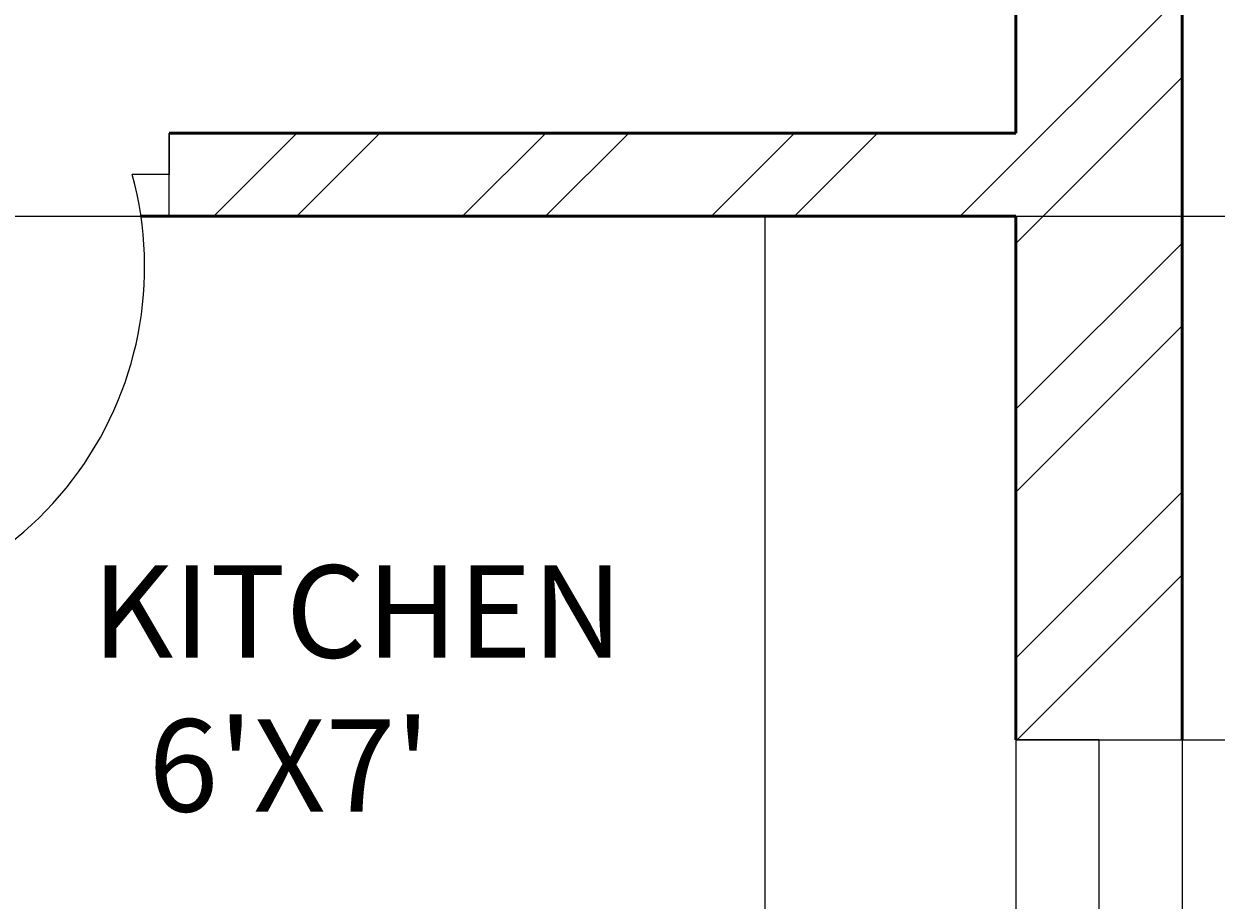
# Model space of a CAD drawing. Units: inches. Extents: x 2310 to 2937, y 1113 to 2410.
# Tile 13 of 23: x 2761 to 2826, y 1845 to 1893. Entities that reach past the tile are written whole.
import ezdxf

# ---------------------------------------------------------------- set-up
doc = ezdxf.new("R2010")
doc.units = ezdxf.units.IN
for name, color, linetype, lineweight in [('A-ANNO-DIMS', 2, 'Continuous', 18), ('A-AREA-IDEN', 7, 'Continuous', 18), ('A-DOOR', 31, 'Continuous', 25), ('A-FLOR-CASE', 7, 'Continuous', 25), ('A-GLAZ', 191, 'Continuous', 20), ('A-WALL', 7, 'Continuous', 50), ('A-WALL-PATT', 85, 'Continuous', 13)]:
    doc.layers.add(name, color=color, linetype=linetype, lineweight=lineweight)
doc.styles.get("Standard").update_dxf_attribs({"font": 'arial.ttf'})
doc.dimstyles.get("Standard").update_dxf_attribs({"dimtxt": 0.18, "dimasz": 0.18, "dimexe": 0.18, "dimexo": 0.0625, "dimgap": 0.09, "dimtad": 0, "dimtih": 1, "dimtoh": 1, "dimdec": 4, "dimzin": 0, "dimdsep": 46, "dimtxsty": 'Standard', "dimcen": 0.09, "dimadec": 0, "dimazin": 0, "dimtfac": 1, "dimtdec": 4, "dimtofl": 0, "dimtmove": 0, "dimatfit": 3, "dimfxl": 1, "dimtolj": 1, "dimtzin": 0, "dimarcsym": 0})

# ---------------------------------------------------------------- blocks, each defined once
blk = doc.blocks.new('WIN-36IN')
for p, q in [((4.5, 36), (0, 36)), ((0, 36), (9, 36)), ((0, 36), (0, 0)), ((4.5, 0), (4.5, 36)), ((9, 36), (9, 0)), ((0, 0), (9, 0)), ((9, 0), (4.5, 0))]:
    blk.add_line(p, q)
blk = doc.blocks.new('*D47')
at = {"layer": 'A-ANNO-DIMS', "color": 0, "lineweight": -2, "transparency": 16777216}
for p, q in [((2824.048, 1909.978), (2858.016, 1909.978)), ((2857.836, 1909.798), (2857.836, 1882.256)), ((2857.836, 1854.35), (2857.836, 1881.893)), ((2824.048, 1854.17), (2858.016, 1854.17))]:
    blk.add_line(p, q, dxfattribs=at)
at = {"layer": 'A-ANNO-DIMS', "color": 0, "transparency": 16777216}
for points in [[(2857.806, 1909.798), (2857.866, 1909.798), (2857.836, 1909.978)], [(2857.806, 1854.35), (2857.866, 1854.35), (2857.836, 1854.17)]]:
    blk.add_solid(points, dxfattribs=at)
at = {"layer": 'Defpoints', "color": 0, "transparency": 16777216}
for p in [(2823.986, 1909.978), (2857.836, 1909.978), (2823.986, 1854.17)]:
    blk.add_point(p, dxfattribs=at)
at = {"layer": 'A-ANNO-DIMS', "color": 0, "transparency": 16777216, "insert": (2857.836, 1882.074), "char_height": 0.18, "attachment_point": 5}
blk.add_mtext('\\A1;55.81', dxfattribs=at)
blk = doc.blocks.new('*D58')
at = {"layer": 'A-ANNO-DIMS', "color": 0, "lineweight": -2, "transparency": 16777216}
for p, q in [((2475.548, 1882.514), (2858.016, 1882.514)), ((2857.836, 1882.334), (2857.836, 1840.446)), ((2857.836, 1798.194), (2857.836, 1840.082)), ((2475.548, 1798.014), (2858.016, 1798.014))]:
    blk.add_line(p, q, dxfattribs=at)
at = {"layer": 'A-ANNO-DIMS', "color": 0, "transparency": 16777216}
for points in [[(2857.806, 1882.334), (2857.866, 1882.334), (2857.836, 1882.514)], [(2857.806, 1798.194), (2857.866, 1798.194), (2857.836, 1798.014)]]:
    blk.add_solid(points, dxfattribs=at)
at = {"layer": 'Defpoints', "color": 0, "transparency": 16777216}
for p in [(2475.486, 1882.514), (2857.836, 1882.514), (2475.486, 1798.014)]:
    blk.add_point(p, dxfattribs=at)
at = {"layer": 'A-ANNO-DIMS', "color": 0, "transparency": 16777216, "insert": (2857.836, 1840.264), "char_height": 0.18, "attachment_point": 5}
blk.add_mtext('\\A1;84.5', dxfattribs=at)

msp = doc.modelspace()

# ---------------------------------------------------------------- hatches: boundary and pattern name
at = {"layer": 'A-WALL-PATT'}
h = msp.add_hatch(dxfattribs=at)
h.set_pattern_fill('ANSI32', color=256)
h.paths.add_polyline_path([(2639.1394, 2356.5139), (2563.662, 2356.5139), (2563.662, 2347.5139), (2606.9859, 2347.5139), (2606.9859, 2210.5139), (2514.2692, 2210.5139), (2514.2692, 2206.0139), (2606.9859, 2206.0139), (2606.9859, 2098.0139), (2602.689, 2098.0139), (2602.689, 2093.5139), (2615.5262, 2093.5139), (2615.5262, 2095.7639), (2615.5262, 2098.0139), (2611.4859, 2098.0139), (2611.4859, 2206.0139), (2703.9391, 2206.0139), (2703.9391, 2208.2639), (2703.9391, 2210.5139), (2611.4859, 2210.5139), (2611.4859, 2347.5139), (2639.1394, 2347.5139)])
h.paths.add_polyline_path([(2823.9859, 2356.5139), (2699.1394, 2356.5139), (2699.1394, 2347.5139), (2738.4859, 2347.5139), (2738.4859, 2343.9266), (2742.9859, 2343.9266), (2742.9859, 2347.5139), (2814.9859, 2347.5139), (2814.9859, 2336.76), (2823.9859, 2336.76)])
h.paths.add_polyline_path([(2823.9859, 2312.76), (2814.9859, 2312.76), (2814.9859, 2299.5139), (2742.9859, 2299.5139), (2742.9859, 2323.0159), (2740.7359, 2323.0159), (2738.4859, 2323.0159), (2738.4859, 2210.5139), (2734.5483, 2210.5139), (2734.5483, 2206.0139), (2746.8769, 2206.0139), (2746.8769, 2208.2639), (2746.8769, 2210.5139), (2742.9859, 2210.5139), (2742.9859, 2295.0139), (2814.9859, 2295.0139), (2814.9859, 2269.8977), (2823.9859, 2269.8977)])
h.paths.add_polyline_path([(2823.9859, 2210.5139), (2823.9859, 2233.8977), (2819.4859, 2233.8977), (2814.9859, 2233.8977), (2814.9859, 2210.5139), (2769.9745, 2210.5139), (2769.9745, 2206.0139), (2814.9859, 2206.0139), (2814.9859, 2178.3027), (2823.9859, 2178.3027)])
h.paths.add_polyline_path([(2823.9859, 2118.3027), (2819.4859, 2118.3027), (2814.9859, 2118.3027), (2814.9859, 2098.0139), (2647.0333, 2098.0139), (2647.0333, 2093.5139), (2814.9859, 2093.5139), (2814.9859, 1999.5139), (2650.6052, 1999.5139), (2650.6052, 1995.0139), (2814.9859, 1995.0139), (2814.9859, 1969.9784), (2823.9859, 1969.9784)])
h.paths.add_polyline_path([(2403.4859, 2093.5139), (2569.9888, 2093.5139), (2569.9888, 2095.7639), (2569.9888, 2098.0139), (2403.4859, 2098.0139), (2403.4859, 2131.7587), (2394.4859, 2131.7587), (2394.4859, 1967.522), (2403.4859, 1967.522), (2403.4859, 1995.0139), (2569.8903, 1995.0139), (2569.8903, 1997.2639), (2569.8903, 1999.5139), (2403.4859, 1999.5139)])
h.paths.add_polyline_path([(2503.662, 2356.5139), (2394.4859, 2356.5139), (2394.4859, 2337.9231), (2398.9859, 2337.9231), (2403.4859, 2337.9231), (2403.4859, 2347.5139), (2475.4859, 2347.5139), (2475.4859, 2343.0384), (2479.9859, 2343.0384), (2479.9859, 2347.5139), (2503.662, 2347.5139)])
h.paths.add_polyline_path([(2498.3065, 1745.5139), (2479.9859, 1745.5139), (2479.9859, 1749.1663), (2477.7359, 1749.1663), (2475.4859, 1749.1663), (2475.4859, 1745.5139), (2403.4859, 1745.5139), (2403.4859, 1753.6409), (2398.9859, 1753.6409), (2394.4859, 1753.6409), (2394.4859, 1736.5139), (2498.3065, 1736.5139), (2498.3065, 1741.0139)])
h.paths.add_polyline_path([(2479.9859, 1882.5139), (2483.9367, 1882.5139), (2483.9367, 1887.0139), (2471.5501, 1887.0139), (2471.5501, 1885.1969), (2471.5501, 1882.5139), (2475.4859, 1882.5139), (2475.4859, 1798.0139), (2403.4859, 1798.0139), (2403.4859, 1828.0433), (2402.2852, 1828.0433), (2394.4859, 1828.0433), (2394.4859, 1777.6409), (2403.4859, 1777.6409), (2403.4859, 1793.5139), (2475.4859, 1793.5139), (2475.4859, 1769.1696), (2479.9859, 1769.1696)])
h.paths.add_polyline_path([(2403.4859, 1907.522), (2398.9859, 1907.522), (2394.4859, 1907.522), (2394.4859, 1864.0433), (2403.4859, 1864.0433), (2403.4859, 1882.5139), (2448.9325, 1882.5139), (2448.9325, 1884.7639), (2448.9325, 1887.0139), (2403.4859, 1887.0139)])
h.paths.add_polyline_path([(2702.2061, 1887.0139), (2611.4859, 1887.0139), (2611.4859, 1995.0139), (2615.6132, 1995.0139), (2615.6132, 1999.5139), (2602.4798, 1999.5139), (2602.4798, 1997.2639), (2602.4798, 1995.0139), (2606.9859, 1995.0139), (2606.9859, 1887.0139), (2516.2443, 1887.0139), (2516.2443, 1884.7639), (2516.2443, 1882.5139), (2606.9859, 1882.5139), (2606.9859, 1745.5139), (2558.3065, 1745.5139), (2558.3065, 1736.5139), (2638.8921, 1736.5139), (2638.8921, 1741.0139), (2638.8921, 1745.5139), (2611.4859, 1745.5139), (2611.4859, 1882.5139), (2702.2061, 1882.5139)])
h.paths.add_polyline_path([(2823.9859, 1909.9784), (2819.4859, 1909.9784), (2814.9859, 1909.9784), (2814.9859, 1887.0139), (2769.144, 1887.0139), (2769.144, 1884.7639), (2769.144, 1882.5139), (2814.9859, 1882.5139), (2814.9859, 1854.1704), (2823.9859, 1854.1704)])
h.paths.add_polyline_path([(2823.9859, 1818.1704), (2819.4859, 1818.1704), (2814.9859, 1818.1704), (2814.9859, 1798.0139), (2742.9859, 1798.0139), (2742.9859, 1882.5139), (2746.805, 1882.5139), (2746.805, 1887.0139), (2733.7334, 1887.0139), (2733.7334, 1884.7639), (2733.7334, 1882.5139), (2738.4859, 1882.5139), (2738.4859, 1771.1728), (2740.7359, 1771.1728), (2742.9859, 1771.1728), (2742.9859, 1793.5139), (2814.9859, 1793.5139), (2814.9859, 1783.6684), (2823.9859, 1783.6684)])
h.paths.add_polyline_path([(2823.9859, 1759.6684), (2814.9859, 1759.6684), (2814.9859, 1745.5139), (2742.9859, 1745.5139), (2742.9859, 1748.9831), (2740.7359, 1748.9831), (2738.4859, 1748.9831), (2738.4859, 1745.5139), (2698.8921, 1745.5139), (2698.8921, 1736.5139), (2823.9859, 1736.5139)])

# ---------------------------------------------------------------- linework, layer by layer
at = {"layer": 'A-DOOR'}
for p, q in [((2769.144, 1882.5139), (2769.144, 1887.0139)), ((2769.144, 1887.0139), (2769.144, 1884.7639)), ((2769.144, 1884.7639), (2767.144, 1884.7639))]:
    msp.add_line(p, q, dxfattribs=at)
msp.add_arc((2748.805, 1879.7705), 19.0066, 270, 15.231482, dxfattribs=at)
at = {"layer": 'A-FLOR-CASE'}
msp.add_line((2801.3852, 1882.5139), (2801.3852, 1812.1659), dxfattribs=at)
at = {"layer": 'A-WALL'}
for p, q in [((2814.9859, 1887.0139), (2814.9859, 1909.9784)), ((2823.9859, 1909.9784), (2823.9859, 1854.1704)), ((2769.144, 1887.0139), (2814.9859, 1887.0139)), ((2767.6126, 1882.5139), (2814.9859, 1882.5139)), ((2814.9859, 1854.1704), (2814.9859, 1882.5139))]:
    msp.add_line(p, q, dxfattribs=at)

# ---------------------------------------------------------------- block references
at = {"layer": 'A-GLAZ'}
msp.add_blockref('WIN-36IN', (2814.9859, 1818.1704), dxfattribs=at)

# ---------------------------------------------------------------- texts
at = {"layer": 'A-AREA-IDEN', "insert": (2761.9054, 1863.6106), "char_height": 5, "attachment_point": 1}
msp.add_mtext_dynamic_manual_height_columns("  KITCHEN\\P    6'X7'", width=98.280022, gutter_width=12.5, heights=[0], dxfattribs=at)

# ---------------------------------------------------------------- dimensions: what is measured, and where the dimension line sits
at = {"layer": 'A-ANNO-DIMS'}
for base, p1, p2, override, picture, middle in [((2857.8359, 1909.9784), (2823.9859, 1854.1704), (2823.9859, 1909.9784), {"dimdec": 2, "dimlfac": 1, "dimrnd": 0, "dimzin": 0, "dimdsep": 46, "dimlunit": 2}, '*D47', (2857.8359, 1882.0744)), ((2857.8359, 1882.5139), (2475.4859, 1798.0139), (2475.4859, 1882.5139), {"dimdec": 1, "dimlfac": 1, "dimrnd": 0, "dimzin": 0, "dimdsep": 46, "dimlunit": 2}, '*D58', (2857.8359, 1840.2639))]:
    dim = msp.add_linear_dim(base=base, p1=p1, p2=p2, angle=90, dimstyle='Standard', override=override, dxfattribs=at)
    dim.commit()
    dim.dimension.update_dxf_attribs({"geometry": picture, "text_midpoint": middle})

doc.saveas('drawing.dxf')
